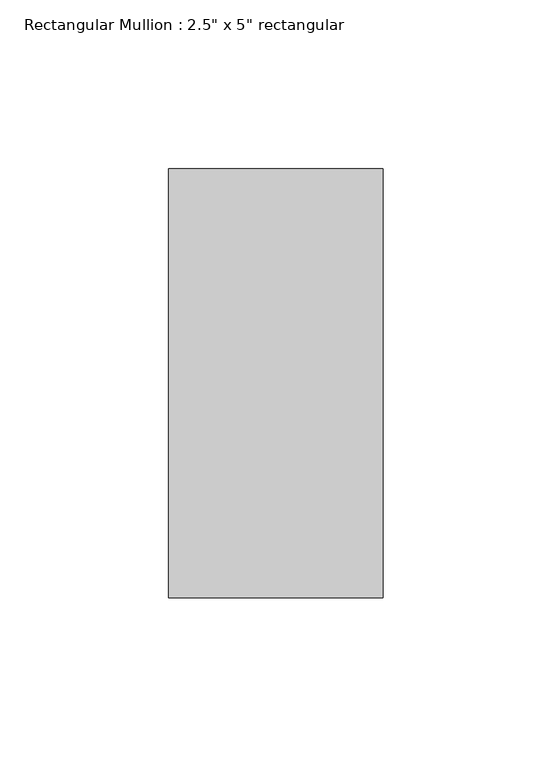
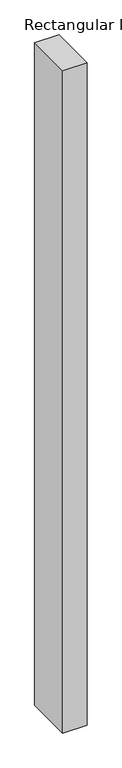
"""IFC4 building model written with IfcOpenShell, lengths in millimetres: member geometry."""

from ifc_helpers import new_model, si_unit, frame, origin, place, context, project, spatial, polyline, outline, extrude, source, transform, mapped, element, save


def member_05d05a14(model_context):
    return source(origin(), model_context, "Body", "SweptSolid", [
        extrude(outline(polyline([(31.75, 63.5), (31.75, -63.5), (-31.75, -63.5), (-31.75, 63.5), (31.75, 63.5)])), frame((0.0, 0.0, -1832.8927429), z_axis=(0.0, 0.0, 1.0), x_axis=(1.0, 0.0, 0.0)), (0.0, 0.0, 1.0), 1832.8927429),
    ])


if __name__ == "__main__":
    model = new_model("IFC4")
    model_context = context("Model", 3, world=origin())
    ifc_project = project(units=[si_unit("LENGTHUNIT", "METRE", prefix="MILLI")], contexts=[model_context])
    site = spatial("IfcSite", under=ifc_project)
    building = spatial("IfcBuilding", under=site)
    placement = place(None, origin())
    member_shape = member_05d05a14(model_context)
    element("IfcMember", 1, ObjectType="Rectangular Mullion : 2.5\" x 5\" rectangular", at=placement, inside=building, context=model_context, shape_type="MappedRepresentation", body=[
        mapped(member_shape, transform((0.0, 0.0, 0.0), x_axis=(1.0, 0.0, 0.0), y_axis=(0.0, 1.0, 0.0), z_axis=(0.0, 0.0, 1.0))),
    ])
    save(model, "model.ifc")

# Revit data of these elements
# Type "Rectangular Mullion : 2.5\" x 5\" rectangular"
#   built-in parameter 1007304 = 0.416667 (stored number, unit not read)
#   built-in parameter 1007301 = 0.104167 (stored number, unit not read)
#   built-in parameter 1007300 = 0.104167 (stored number, unit not read)
# Element 1 (IfcMember, "Rectangular Mullion : 2.5\" x 5\" rectangular")
#   Materials on its faces: "Aluminum"
# Materials
#   "Aluminum": class "Metal", colour RGB 247 247 247, transparency 0, Description = "Aluminum 6061", Cost = 0
